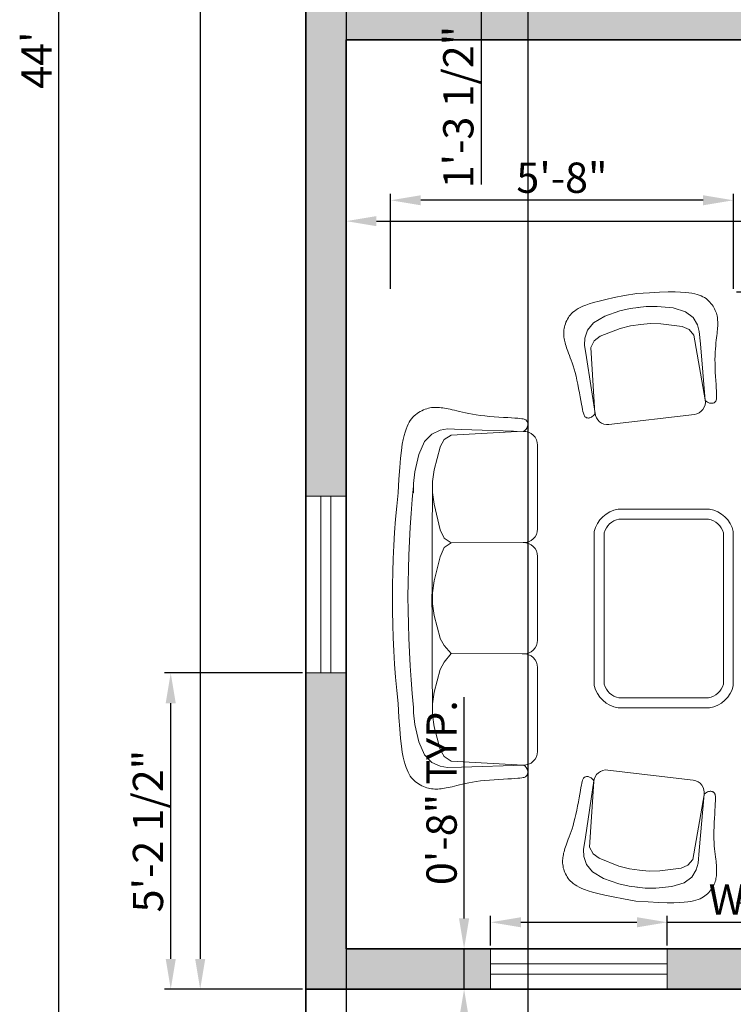
# Model space of a CAD drawing. Units: inches. Extents: x 2129 to 3258, y 1851 to 3021.
# Tile 2 of 10: x 2129 to 2271, y 1956 to 2151. Entities that reach past the tile are written whole.
import ezdxf

# ---------------------------------------------------------------- set-up
doc = ezdxf.new("R2010")
doc.units = ezdxf.units.IN
for name, color, linetype, lineweight in [('A-ANNO-DIMS', 2, 'Continuous', 18), ('A-FURN', 8, 'Continuous', 18), ('A-GLAZ', 4, 'Continuous', 18), ('A-WALL', 7, 'Continuous', 35)]:
    doc.layers.add(name, color=color, linetype=linetype, lineweight=lineweight)
doc.layers.add('A-WALL-PATT', color=32, linetype='Continuous', lineweight=13, true_color=0xcd6928)
doc.styles.get("Standard").update_dxf_attribs({"font": 'arial.ttf'})
doc.dimstyles.new('ISO-25', dxfattribs={"dimtxt": 6, "dimasz": 6, "dimexe": 1.25, "dimexo": 0.625, "dimtad": 1, "dimdec": 1, "dimlunit": 3, "dimtxsty": 'Standard', "dimcen": 2.5, "dimclrd": 5, "dimclre": 5, "dimadec": 0, "dimazin": 0, "dimtfac": 1, "dimtdec": 1, "dimtmove": 0, "dimatfit": 3, "dimfxl": 1, "dimarcsym": 0})

# ---------------------------------------------------------------- blocks, each defined once
blk = doc.blocks.new('sofa arrangement 10')
for p, q in [((-548, 1633.4), (-478.2, 1637.4)), ((651.3, 1633.4), (581.5, 1637.4)), ((-833.9, 1581.8), (-823.7, 1587.2)), ((-823.7, 1587.2), (-812.1, 1592.5)), ((-812.1, 1592.5), (-799.1, 1597.5)), ((-799.1, 1597.5), (-784.4, 1602.4)), ((-784.4, 1602.4), (-767.6, 1607.2)), ((-767.6, 1607.2), (-747.5, 1611.8)), ((-747.5, 1611.8), (-722.8, 1616.4)), ((-722.8, 1616.4), (-691.9, 1620.8)), ((-691.9, 1620.8), (-653.4, 1625.1)), ((-653.4, 1625.1), (-605.9, 1629.3)), ((-605.9, 1629.3), (-548, 1633.4)), ((709.2, 1629.3), (651.3, 1633.4)), ((756.7, 1625.1), (709.2, 1629.3)), ((795.2, 1620.8), (756.7, 1625.1)), ((826.1, 1616.4), (795.2, 1620.8)), ((850.9, 1611.8), (826.1, 1616.4)), ((870.9, 1607.2), (850.9, 1611.8)), ((887.7, 1602.4), (870.9, 1607.2)), ((902.4, 1597.5), (887.7, 1602.4)), ((915.5, 1592.5), (902.4, 1597.5)), ((927, 1587.2), (915.5, 1592.5)), ((937.2, 1581.8), (927, 1587.2)), ((-882.6, 1534.1), (-877.2, 1542)), ((-877.2, 1542), (-871.4, 1549.5)), ((-871.4, 1549.5), (-865.1, 1556.8)), ((-865.1, 1556.8), (-858.4, 1563.6)), ((-858.4, 1563.6), (-851.1, 1570)), ((-851.1, 1570), (-843, 1576)), ((-843, 1576), (-833.9, 1581.8)), ((-670.8, 1533.8), (-584, 1552.9)), ((-584, 1552.9), (-524.7, 1559.2)), ((-524.7, 1559.2), (-497.4, 1559.2)), ((628.1, 1559.2), (581.5, 1559.2)), ((607.1, 1559.2), (585.6, 1559.2)), ((687.3, 1552.9), (628.1, 1559.2)), ((774.1, 1533.8), (687.3, 1552.9)), ((946.3, 1576), (937.2, 1581.8)), ((954.4, 1570), (946.3, 1576)), ((961.8, 1563.6), (954.4, 1570)), ((968.5, 1556.8), (961.8, 1563.6)), ((974.8, 1549.5), (968.5, 1556.8)), ((980.6, 1542), (974.8, 1549.5)), ((985.9, 1534.1), (980.6, 1542)), ((-904.1, 1484.8), (-901.8, 1492.9)), ((-901.8, 1492.9), (-899, 1501.2)), ((-899, 1501.2), (-895.7, 1509.5)), ((-895.7, 1509.5), (-891.8, 1517.8)), ((-891.8, 1517.8), (-887.5, 1526)), ((-887.5, 1526), (-882.6, 1534.1)), ((-774.5, 1468.3), (-736.4, 1504.2)), ((-736.4, 1504.2), (-670.8, 1533.8)), ((839.7, 1504.2), (774.1, 1533.8)), ((877.8, 1468.3), (839.7, 1504.2)), ((990.8, 1526), (985.9, 1534.1)), ((995.2, 1517.8), (990.8, 1526)), ((999, 1509.5), (995.2, 1517.8)), ((1002.4, 1501.2), (999, 1509.5)), ((1005.2, 1492.9), (1002.4, 1501.2)), ((1007.4, 1484.8), (1005.2, 1492.9)), ((-908.3, 1445.1), (-908.2, 1453)), ((-908, 1437.2), (-908.3, 1445.1)), ((-908.2, 1453), (-907.8, 1460.9)), ((-907.5, 1429.1), (-908, 1437.2)), ((-907.8, 1460.9), (-907, 1468.8)), ((-907, 1468.8), (-905.8, 1476.8)), ((-905.8, 1476.8), (-904.1, 1484.8)), ((-793.5, 1426), (-774.5, 1468.3)), ((-594.6, 1455.6), (-708.9, 1426)), ((-535.3, 1464), (-594.6, 1455.6)), ((-478.2, 1464), (-535.3, 1464)), ((-421, 1455.6), (-480.3, 1464)), ((-480.3, 1464), (-478.2, 1464)), ((-306.7, 1426), (-421, 1455.6)), ((-149.4, 1426), (-35.1, 1455.6)), ((-35.1, 1455.6), (24.1, 1464)), ((24.1, 1464), (77.1, 1464)), ((77.1, 1464), (79.2, 1464)), ((79.2, 1464), (138.5, 1455.6)), ((138.5, 1455.6), (260.8, 1426)), ((896.9, 1426), (877.8, 1468.3)), ((1009.1, 1476.8), (1007.4, 1484.8)), ((1010.4, 1468.8), (1009.1, 1476.8)), ((1011.2, 1460.9), (1010.4, 1468.8)), ((1010.8, 1429.1), (1011.4, 1437.2)), ((1011.6, 1453), (1011.2, 1460.9)), ((1011.4, 1437.2), (1011.6, 1445.1)), ((1011.6, 1445.1), (1011.6, 1453)), ((-906.7, 1421), (-907.5, 1429.1)), ((-905.7, 1412.7), (-906.7, 1421)), ((-904.4, 1404.1), (-905.7, 1412.7)), ((-902.8, 1395.1), (-904.4, 1404.1)), ((-901, 1385.6), (-902.8, 1395.1)), ((-799.9, 1387.9), (-793.5, 1426)), ((-797.8, 1318.1), (-799.9, 1387.9)), ((-744.9, 1404.8), (-768.1, 1371)), ((-708.9, 1426), (-744.9, 1404.8)), ((-306.7, 1426), (-270.7, 1404.8)), ((-270.7, 1404.8), (-226.6, 1371)), ((-186.6, 1404.8), (-226.6, 1371)), ((-150.6, 1426), (-186.6, 1404.8)), ((260.8, 1426), (306.7, 1404.8)), ((813.4, 1426), (849.4, 1404.8)), ((849.4, 1404.8), (872.7, 1371)), ((849.4, 1404.8), (872.7, 1371)), ((903.2, 1387.9), (896.9, 1426)), ((901.1, 1318.1), (903.2, 1387.9)), ((1004.4, 1385.6), (1006.2, 1395.1)), ((1006.2, 1395.1), (1007.7, 1404.1)), ((1007.7, 1404.1), (1009, 1412.7)), ((1009, 1412.7), (1010, 1421)), ((1010, 1421), (1010.8, 1429.1)), ((-898.9, 1375.6), (-901, 1385.6)), ((-896.5, 1364.8), (-898.9, 1375.6)), ((-893.7, 1353.4), (-896.5, 1364.8)), ((-890.7, 1341), (-893.7, 1353.4)), ((-887.4, 1327.7), (-890.7, 1341)), ((-768.1, 1371), (-787.5, 1008.1)), ((-226.6, 1371), (-228.1, 1008.1)), ((-226.6, 1371), (-228.1, 1008.1)), ((872.7, 1371), (892.1, 1008.1)), ((990.7, 1327.7), (994, 1341)), ((994, 1341), (997.1, 1353.4)), ((997.1, 1353.4), (999.8, 1364.8)), ((999.8, 1364.8), (1002.2, 1375.6)), ((1002.2, 1375.6), (1004.4, 1385.6)), ((-883.9, 1313.4), (-887.4, 1327.7)), ((-880.4, 1297.9), (-883.9, 1313.4)), ((-876.9, 1281.2), (-880.4, 1297.9)), ((-787.6, 1004.4), (-797.8, 1318.1)), ((891, 1004.4), (901.1, 1318.1)), ((980.3, 1281.2), (983.7, 1297.9)), ((983.7, 1297.9), (987.3, 1313.4)), ((987.3, 1313.4), (990.7, 1327.7)), ((-873.6, 1263.2), (-876.9, 1281.2)), ((-870.4, 1243.8), (-873.6, 1263.2)), ((-867.6, 1222.9), (-870.4, 1243.8)), ((971, 1222.9), (973.8, 1243.8)), ((973.8, 1243.8), (976.9, 1263.2)), ((976.9, 1263.2), (980.3, 1281.2)), ((-865.2, 1200.6), (-867.6, 1222.9)), ((-863, 1177.2), (-865.2, 1200.6)), ((966.4, 1177.2), (968.5, 1200.6)), ((968.5, 1200.6), (971, 1222.9)), ((-861.2, 1153.4), (-863, 1177.2)), ((-859.7, 1129.8), (-861.2, 1153.4)), ((963, 1129.8), (964.6, 1153.4)), ((964.6, 1153.4), (966.4, 1177.2)), ((-858.3, 1107), (-859.7, 1129.8)), ((-857.1, 1085.6), (-858.3, 1107)), ((960.4, 1085.6), (961.7, 1107)), ((961.7, 1107), (963, 1129.8)), ((-856, 1066.1), (-857.1, 1085.6)), ((-854.9, 1049.1), (-856, 1066.1)), ((-853.9, 1035.2), (-854.9, 1049.1)), ((957.2, 1035.2), (958.3, 1049.1)), ((958.3, 1049.1), (959.3, 1066.1)), ((959.3, 1066.1), (960.4, 1085.6)), ((-852.8, 1024), (-853.9, 1035.2)), ((-851.7, 1015.2), (-852.8, 1024)), ((-850.5, 1008.5), (-851.7, 1015.2)), ((-849.3, 1003.4), (-850.5, 1008.5)), ((-848, 999.6), (-849.3, 1003.4)), ((-846.6, 996.8), (-848, 999.6)), ((-845, 994.5), (-846.6, 996.8)), ((-843.4, 992.5), (-845, 994.5)), ((-841.6, 990.7), (-843.4, 992.5)), ((-839.6, 989.1), (-841.6, 990.7)), ((-799.3, 993.5), (-804.6, 989.9)), ((-793.6, 998.3), (-799.3, 993.5)), ((-787.6, 1004.4), (-793.6, 998.3)), ((-786.9, 1011.2), (-787.4, 1011.2)), ((-787.4, 1010.4), (-786.9, 1011.2)), ((-229.1, 1010.4), (-228.7, 1011.2)), ((-228.7, 1011.2), (-229.1, 1011.2)), ((-228.7, 1011.2), (-228.2, 1011.2)), ((-228.2, 1010.4), (-228.7, 1011.2)), ((890.3, 1011.2), (890.7, 1011.2)), ((890.8, 1010.4), (890.3, 1011.2)), ((891, 1004.4), (897, 998.3)), ((897, 998.3), (902.6, 993.5)), ((902.6, 993.5), (907.9, 989.9)), ((942.9, 989.1), (944.9, 990.7)), ((944.9, 990.7), (946.7, 992.5)), ((946.7, 992.5), (948.4, 994.5)), ((948.4, 994.5), (949.9, 996.8)), ((949.9, 996.8), (951.3, 999.6)), ((951.3, 999.6), (952.6, 1003.4)), ((952.6, 1003.4), (953.9, 1008.5)), ((953.9, 1008.5), (955, 1015.2)), ((955, 1015.2), (956.1, 1024)), ((956.1, 1024), (957.2, 1035.2)), ((-837.4, 987.7), (-839.6, 989.1)), ((-834.9, 986.6), (-837.4, 987.7)), ((-832.2, 985.7), (-834.9, 986.6)), ((-829.3, 985), (-832.2, 985.7)), ((-826, 984.6), (-829.3, 985)), ((-822.4, 984.5), (-826, 984.6)), ((-818.4, 984.8), (-822.4, 984.5)), ((-814.2, 985.7), (-818.4, 984.8)), ((-809.6, 987.4), (-814.2, 985.7)), ((-804.6, 989.9), (-809.6, 987.4)), ((907.9, 989.9), (912.9, 987.4)), ((912.9, 987.4), (917.5, 985.7)), ((917.5, 985.7), (921.8, 984.8)), ((921.8, 984.8), (925.7, 984.5)), ((925.7, 984.5), (929.3, 984.6)), ((929.3, 984.6), (932.6, 985)), ((932.6, 985), (935.6, 985.7)), ((935.6, 985.7), (938.3, 986.6)), ((938.3, 986.6), (940.7, 987.7)), ((940.7, 987.7), (942.9, 989.1)), ((-718.5, 935.3), (-297.1, 935.3)), ((262.4, 935.3), (-159, 935.3)), ((-1335.3, 794.4), (-1343, 790.4)), ((-1327.5, 797.9), (-1335.3, 794.4)), ((-1319.6, 801), (-1327.5, 797.9)), ((-1311.7, 803.6), (-1319.6, 801)), ((-1303.8, 805.7), (-1311.7, 803.6)), ((-1296.1, 807.3), (-1303.8, 805.7)), ((-1288.5, 808.5), (-1296.1, 807.3)), ((-1281.1, 809.2), (-1288.5, 808.5)), ((-1273.7, 809.4), (-1281.1, 809.2)), ((-1266.5, 809.3), (-1273.7, 809.4)), ((-1259.4, 808.8), (-1266.5, 809.3)), ((-1252.2, 808), (-1259.4, 808.8)), ((-1245.1, 806.9), (-1252.2, 808)), ((-1237.9, 805.5), (-1245.1, 806.9)), ((-1230.6, 804), (-1237.9, 805.5)), ((-1223.2, 802.1), (-1230.6, 804)), ((-1215.6, 800.1), (-1223.2, 802.1)), ((-1207.6, 797.7), (-1215.6, 800.1)), ((-1199.3, 795), (-1207.6, 797.7)), ((-1190.4, 792), (-1199.3, 795)), ((1320.4, 792.1), (1328.3, 794.5)), ((1328.3, 794.5), (1336, 796.6)), ((1336, 796.6), (1343.4, 798.4)), ((1343.4, 798.4), (1350.6, 800)), ((1350.6, 800), (1357.8, 801.3)), ((1357.8, 801.3), (1365, 802.4)), ((1365, 802.4), (1372.1, 803.2)), ((1372.1, 803.2), (1379.3, 803.7)), ((1379.3, 803.7), (1386.5, 803.8)), ((1386.5, 803.8), (1393.8, 803.6)), ((1393.8, 803.6), (1401.3, 802.9)), ((1401.3, 802.9), (1408.8, 801.8)), ((1408.8, 801.8), (1416.6, 800.1)), ((1416.6, 800.1), (1424.5, 798)), ((1424.5, 798), (1432.4, 795.4)), ((1432.4, 795.4), (1440.3, 792.4)), ((-1389.6, 746.9), (-1395.6, 737.1)), ((-1383.6, 755.6), (-1389.6, 746.9)), ((-1377.4, 763.2), (-1383.6, 755.6)), ((-1371.1, 769.8), (-1377.4, 763.2)), ((-1364.5, 775.8), (-1371.1, 769.8)), ((-1357.6, 781.1), (-1364.5, 775.8)), ((-1350.5, 786), (-1357.6, 781.1)), ((-1343, 790.4), (-1350.5, 786)), ((-1181, 788.7), (-1190.4, 792)), ((-1171, 784.9), (-1181, 788.7)), ((-1160.1, 780.9), (-1171, 784.9)), ((-1148.5, 776.4), (-1160.1, 780.9)), ((-1135.9, 771.8), (-1148.5, 776.4)), ((-1122.4, 766.9), (-1135.9, 771.8)), ((-1107.7, 762), (-1122.4, 766.9)), ((-1091.8, 757), (-1107.7, 762)), ((-1074.6, 752.1), (-1091.8, 757)), ((-1056, 747.3), (-1074.6, 752.1)), ((-1036.1, 742.7), (-1056, 747.3)), ((1168.8, 741.7), (1187.4, 746.5)), ((1187.4, 746.5), (1204.5, 751.5)), ((1204.5, 751.5), (1220.4, 756.4)), ((1220.4, 756.4), (1235.1, 761.4)), ((1235.1, 761.4), (1248.7, 766.2)), ((1248.7, 766.2), (1261.3, 770.9)), ((1261.3, 770.9), (1272.9, 775.3)), ((1272.9, 775.3), (1283.7, 779.4)), ((1283.7, 779.4), (1293.8, 783.1)), ((1293.8, 783.1), (1303.2, 786.4)), ((1303.2, 786.4), (1312, 789.4)), ((1312, 789.4), (1320.4, 792.1)), ((1440.3, 792.4), (1448.1, 788.8)), ((1448.1, 788.8), (1455.8, 784.8)), ((1455.8, 784.8), (1463.2, 780.4)), ((1463.2, 780.4), (1470.4, 775.5)), ((1470.4, 775.5), (1477.3, 770.2)), ((1477.3, 770.2), (1483.8, 764.3)), ((1483.8, 764.3), (1490.2, 757.6)), ((1490.2, 757.6), (1496.3, 750)), ((1496.3, 750), (1502.4, 741.4)), ((-1413.7, 698.5), (-1420, 680.9)), ((-1407.6, 713.1), (-1413.7, 698.5)), ((-1401.6, 725.9), (-1407.6, 713.1)), ((-1395.6, 737.1), (-1401.6, 725.9)), ((-1247.3, 702.4), (-1287.6, 689.7)), ((-1212.3, 704), (-1247.3, 702.4)), ((-1149.5, 694.5), (-1212.3, 704)), ((-867.4, 651.5), (-1149.5, 694.5)), ((-1015.2, 738.3), (-1036.1, 742.7)), ((-994, 734.1), (-1015.2, 738.3)), ((-972.9, 730.1), (-994, 734.1)), ((-952.4, 726.4), (-972.9, 730.1)), ((-933.2, 723), (-952.4, 726.4)), ((-915.7, 719.9), (-933.2, 723)), ((-900.5, 717.1), (-915.7, 719.9)), ((-888.1, 714.6), (-900.5, 717.1)), ((-878.1, 712.5), (-888.1, 714.6)), ((-870.3, 710.5), (-878.1, 712.5)), ((-864.3, 708.7), (-870.3, 710.5)), ((-859.9, 707.1), (-864.3, 708.7)), ((-856.6, 705.5), (-859.9, 707.1)), ((-854.2, 703.9), (-856.6, 705.5)), ((-852.3, 702.3), (-854.2, 703.9)), ((-850.6, 700.6), (-852.3, 702.3)), ((-849.2, 698.7), (-850.6, 700.6)), ((-848, 696.8), (-849.2, 698.7)), ((-847, 694.6), (-848, 696.8)), ((-846.2, 692.3), (-847, 694.6)), ((962, 693.2), (963.4, 695)), ((963.4, 695), (965, 696.7)), ((965, 696.7), (966.9, 698.3)), ((966.9, 698.3), (969.3, 699.9)), ((969.3, 699.9), (972.6, 701.5)), ((972.6, 701.5), (977.1, 703.2)), ((977.1, 703.2), (983, 704.9)), ((983, 704.9), (990.8, 706.9)), ((990.8, 706.9), (1000.8, 709.1)), ((1000.8, 709.1), (1013.3, 711.5)), ((1013.3, 711.5), (1028.5, 714.3)), ((1028.5, 714.3), (1045.9, 717.4)), ((1045.9, 717.4), (1065.2, 720.8)), ((1065.2, 720.8), (1085.6, 724.5)), ((1085.6, 724.5), (1106.7, 728.5)), ((1106.7, 728.5), (1128, 732.7)), ((1128, 732.7), (1148.9, 737.1)), ((1148.9, 737.1), (1168.8, 741.7)), ((1262.2, 689), (1325, 698.4)), ((1325, 698.4), (1360.1, 696.8)), ((1360.1, 696.8), (1400.3, 684.2)), ((1502.4, 741.4), (1508.4, 731.5)), ((1508.4, 731.5), (1514.3, 720.3)), ((1514.3, 720.3), (1520.3, 707.5)), ((1520.3, 707.5), (1526.4, 692.9)), ((-1426.8, 659), (-1434.1, 631.6)), ((-1420, 680.9), (-1426.8, 659)), ((-1324.1, 659.2), (-1357.9, 603.2)), ((-1287.6, 689.7), (-1324.1, 659.2)), ((-1256.4, 625.9), (-1233.5, 656.1)), ((-1233.5, 656.1), (-1200.4, 673.5)), ((-1200.4, 673.5), (-870.8, 651.8)), ((-873.7, 651.6), (-873.6, 652)), ((-872.9, 652), (-873.7, 651.6)), ((-867.4, 651.5), (-861.2, 656.3)), ((-861.2, 656.3), (-856.3, 660.9)), ((-856.3, 660.9), (-852.5, 665.3)), ((-852.5, 665.3), (-849.7, 669.5)), ((-849.7, 669.5), (-847.7, 673.5)), ((-847.7, 673.5), (-846.4, 677.2)), ((-846.4, 677.2), (-845.7, 680.8)), ((-845.7, 689.8), (-846.2, 692.3)), ((-845.4, 687), (-845.7, 689.8)), ((-845.7, 680.8), (-845.4, 684)), ((-845.4, 684), (-845.4, 687)), ((958.2, 681.5), (958.5, 684.2)), ((958.2, 678.5), (958.2, 681.5)), ((958.5, 675.2), (958.2, 678.5)), ((958.5, 684.2), (959, 686.7)), ((959.2, 671.7), (958.5, 675.2)), ((959, 686.7), (959.7, 689.1)), ((960.5, 667.9), (959.2, 671.7)), ((959.7, 689.1), (960.7, 691.2)), ((962.4, 663.9), (960.5, 667.9)), ((960.7, 691.2), (962, 693.2)), ((965.2, 659.7), (962.4, 663.9)), ((969, 655.3), (965.2, 659.7)), ((974, 650.7), (969, 655.3)), ((980.2, 646), (974, 650.7)), ((980.2, 646), (1262.2, 689)), ((1313.2, 667.9), (983.5, 646.3)), ((985.6, 646.4), (986.4, 646.1)), ((986.4, 646.1), (986.4, 646.5)), ((1346.2, 650.6), (1313.2, 667.9)), ((1369.2, 620.4), (1346.2, 650.6)), ((1400.3, 684.2), (1436.9, 653.6)), ((1436.9, 653.6), (1470.7, 597.6)), ((1526.4, 692.9), (1532.8, 675.3)), ((1532.8, 675.3), (1539.6, 653.4)), ((1539.6, 653.4), (1546.9, 626)), ((-1442.2, 597.3), (-1451.1, 554.9)), ((-1434.1, 631.6), (-1442.2, 597.3)), ((-1357.9, 603.2), (-1384.5, 526.9)), ((-1295.5, 526), (-1256.4, 625.9)), ((1408.3, 520.4), (1369.2, 620.4)), ((1470.7, 597.6), (1497.2, 521.3)), ((1546.9, 626), (1554.9, 591.7)), ((-1451.1, 554.9), (-1461.1, 503.1)), ((-812.5, 581.7), (-863.9, 151.6)), ((925.2, 576.1), (976.6, 146.1)), ((1554.9, 591.7), (1563.9, 549.3)), ((1563.9, 549.3), (1573.8, 497.5)), ((-1461.1, 503.1), (-1472.2, 440.5)), ((-1384.5, 526.9), (-1396.6, 474.1)), ((-1309.5, 473.4), (-1295.5, 526)), ((1422.3, 467.8), (1408.3, 520.4)), ((1497.2, 521.3), (1509.4, 468.5)), ((1573.8, 497.5), (1584.9, 434.9)), ((-1396.6, 474.1), (-1401.6, 432.1)), ((-1315.7, 421.8), (-1309.5, 473.4)), ((1428.5, 416.2), (1422.3, 467.8)), ((1509.4, 468.5), (1514.4, 426.5)), ((-1476, 378.3), (-1472.2, 440.5)), ((-1406.2, 393.7), (-1401.2, 435.7)), ((-1321.4, 374), (-1315.7, 421.8)), ((1434.2, 368.5), (1428.5, 416.2)), ((1519, 388.1), (1513.9, 430.2)), ((1588.7, 372.7), (1584.9, 434.9)), ((-1478.4, 326.5), (-1476, 378.3)), ((-1406.9, 339.5), (-1406.2, 393.7)), ((-1320.2, 319.6), (-1321.4, 374)), ((1432.9, 314.1), (1434.2, 368.5)), ((1519.6, 334), (1519, 388.1)), ((1591.2, 320.9), (1588.7, 372.7)), ((-1479.7, 283.8), (-1478.4, 326.5)), ((-1399.1, 259.2), (-1406.9, 339.5)), ((-1305.8, 213.3), (-1320.2, 319.6)), ((1418.5, 207.7), (1432.9, 314.1)), ((1511.8, 253.6), (1519.6, 334)), ((1592.4, 278.2), (1591.2, 320.9)), ((-1479.9, 249.1), (-1479.7, 283.8)), ((-1479.2, 220.9), (-1479.9, 249.1)), ((-1379.4, 196.7), (-1399.1, 259.2)), ((1492.2, 191.2), (1511.8, 253.6)), ((1592.6, 243.5), (1592.4, 278.2)), ((-1477.7, 198.2), (-1479.2, 220.9)), ((-1475.7, 179.7), (-1477.7, 198.2)), ((-1290.6, 178.5), (-1305.8, 213.3)), ((1403.3, 172.9), (1418.5, 207.7)), ((1590.5, 192.7), (1591.9, 215.4)), ((1591.9, 215.4), (1592.6, 243.5)), ((-1473.2, 164), (-1475.7, 179.7)), ((-1470.4, 150.2), (-1473.2, 164)), ((-1467.2, 137.9), (-1470.4, 150.2)), ((-1351.1, 158.5), (-1379.4, 196.7)), ((-1314.9, 136.7), (-1351.1, 158.5)), ((-1262.5, 153.8), (-1290.6, 178.5)), ((-937.1, 97.2), (-1262.5, 153.8)), ((1375.3, 148.3), (1403.3, 172.9)), ((1427.7, 131.1), (1463.8, 152.9)), ((1463.8, 152.9), (1492.2, 191.2)), ((1583.1, 144.6), (1586, 158.4)), ((1586, 158.4), (1588.4, 174.1)), ((1588.4, 174.1), (1590.5, 192.7)), ((-1463.7, 126.9), (-1467.2, 137.9)), ((-1459.9, 117.1), (-1463.7, 126.9)), ((-1455.7, 108.3), (-1459.9, 117.1)), ((-1451.1, 100.3), (-1455.7, 108.3)), ((-1446.1, 93), (-1451.1, 100.3)), ((-1281.3, 126.9), (-1314.9, 136.7)), ((-1218, 121.2), (-1281.3, 126.9)), ((-933.8, 96.5), (-1218, 121.2)), ((1046.5, 91), (1330.8, 115.7)), ((1049.8, 91.6), (1375.3, 148.3)), ((1330.8, 115.7), (1394, 121.3)), ((1394, 121.3), (1427.7, 131.1)), ((1563.9, 94.7), (1568.5, 102.7)), ((1568.5, 102.7), (1572.7, 111.5)), ((1572.7, 111.5), (1576.5, 121.3)), ((1576.5, 121.3), (1580, 132.3)), ((1580, 132.3), (1583.1, 144.6)), ((-1440.7, 86.2), (-1446.1, 93)), ((-1434.9, 79.7), (-1440.7, 86.2)), ((-1428.7, 73.7), (-1434.9, 79.7)), ((-1422.2, 68), (-1428.7, 73.7)), ((-1415.4, 62.7), (-1422.2, 68)), ((-1408.4, 57.9), (-1415.4, 62.7)), ((-1401.4, 53.5), (-1408.4, 57.9)), ((-1394.2, 49.6), (-1401.4, 53.5)), ((-1387.1, 46.2), (-1394.2, 49.6)), ((-933.8, 96.5), (-928.9, 90.5)), ((-928.9, 90.5), (-925.1, 84.8)), ((-924.1, 49.9), (-925.5, 48)), ((-925.1, 84.8), (-922.5, 79.7)), ((-922.8, 51.9), (-924.1, 49.9)), ((-921.7, 54.3), (-922.8, 51.9)), ((-922.5, 79.7), (-920.7, 74.9)), ((-920.8, 56.9), (-921.7, 54.3)), ((-920.1, 59.8), (-920.8, 56.9)), ((-920.7, 74.9), (-919.8, 70.6)), ((-919.6, 63), (-920.1, 59.8)), ((-919.8, 70.6), (-919.4, 66.6)), ((-919.4, 66.6), (-919.6, 63)), ((1032.5, 65), (1032.2, 61)), ((1032.2, 61), (1032.3, 57.5)), ((1032.3, 57.5), (1032.8, 54.2)), ((1033.5, 69.3), (1032.5, 65)), ((1032.8, 54.2), (1033.5, 51.3)), ((1035.2, 74.1), (1033.5, 69.3)), ((1033.5, 51.3), (1034.4, 48.7)), ((1037.9, 79.3), (1035.2, 74.1)), ((1041.6, 84.9), (1037.9, 79.3)), ((1046.5, 91), (1041.6, 84.9)), ((1514.1, 47.9), (1521.2, 52.3)), ((1521.2, 52.3), (1528.2, 57.2)), ((1528.2, 57.2), (1534.9, 62.4)), ((1534.9, 62.4), (1541.4, 68.1)), ((1541.4, 68.1), (1547.6, 74.2)), ((1547.6, 74.2), (1553.5, 80.6)), ((1553.5, 80.6), (1558.9, 87.4)), ((1558.9, 87.4), (1563.9, 94.7)), ((-1380, 43.3), (-1387.1, 46.2)), ((-1372.9, 40.9), (-1380, 43.3)), ((-1365.9, 38.9), (-1372.9, 40.9)), ((-1358.8, 37.3), (-1365.9, 38.9)), ((-1351.7, 36.1), (-1358.8, 37.3)), ((-1344.6, 35.2), (-1351.7, 36.1)), ((-1337.4, 34.6), (-1344.6, 35.2)), ((-1330.1, 34.2), (-1337.4, 34.6)), ((-1322.7, 34), (-1330.1, 34.2)), ((-1315, 34.1), (-1322.7, 34)), ((-1307.1, 34.3), (-1315, 34.1)), ((-1298.8, 34.7), (-1307.1, 34.3)), ((-1290.1, 35.3), (-1298.8, 34.7)), ((-1280.8, 36.2), (-1290.1, 35.3)), ((-1270.9, 37.2), (-1280.8, 36.2)), ((-1260.2, 38.4), (-1270.9, 37.2)), ((-1248.7, 39.9), (-1260.2, 38.4)), ((-1236.4, 41.4), (-1248.7, 39.9)), ((-1223.1, 43), (-1236.4, 41.4)), ((-1208.7, 44.5), (-1223.1, 43)), ((-1193.3, 45.8), (-1208.7, 44.5)), ((-1176.7, 46.9), (-1193.3, 45.8)), ((-1158.8, 47.6), (-1176.7, 46.9)), ((-1139.6, 47.9), (-1158.8, 47.6)), ((-1119.2, 47.7), (-1139.6, 47.9)), ((-1097.9, 47.1), (-1119.2, 47.7)), ((-1076.2, 46.2), (-1097.9, 47.1)), ((-1054.7, 45), (-1076.2, 46.2)), ((-1034, 43.8), (-1054.7, 45)), ((-1014.5, 42.6), (-1034, 43.8)), ((-996.8, 41.5), (-1014.5, 42.6)), ((-981.4, 40.6), (-996.8, 41.5)), ((-968.7, 40.1), (-981.4, 40.6)), ((-958.5, 39.9), (-968.7, 40.1)), ((-950.4, 39.9), (-958.5, 39.9)), ((-944.2, 40.2), (-950.4, 39.9)), ((-939.5, 40.8), (-944.2, 40.2)), ((-936, 41.6), (-939.5, 40.8)), ((-933.2, 42.5), (-936, 41.6)), ((-931, 43.7), (-933.2, 42.5)), ((-929, 44.9), (-931, 43.7)), ((-927.2, 46.4), (-929, 44.9)), ((-925.5, 48), (-927.2, 46.4)), ((1034.4, 48.7), (1035.5, 46.4)), ((1035.5, 46.4), (1036.8, 44.3)), ((1036.8, 44.3), (1038.3, 42.4)), ((1038.3, 42.4), (1039.9, 40.8)), ((1039.9, 40.8), (1041.8, 39.4)), ((1041.8, 39.4), (1043.8, 38.1)), ((1043.8, 38.1), (1046, 37)), ((1046, 37), (1048.7, 36)), ((1048.7, 36), (1052.3, 35.2)), ((1052.3, 35.2), (1057, 34.7)), ((1057, 34.7), (1063.2, 34.3)), ((1063.2, 34.3), (1071.2, 34.3)), ((1071.2, 34.3), (1081.4, 34.5)), ((1081.4, 34.5), (1094.2, 35.1)), ((1094.2, 35.1), (1109.6, 35.9)), ((1109.6, 35.9), (1127.3, 37)), ((1127.3, 37), (1146.8, 38.2)), ((1146.8, 38.2), (1167.5, 39.5)), ((1167.5, 39.5), (1189, 40.6)), ((1189, 40.6), (1210.6, 41.5)), ((1210.6, 41.5), (1231.9, 42.2)), ((1231.9, 42.2), (1252.4, 42.4)), ((1252.4, 42.4), (1271.6, 42.1)), ((1271.6, 42.1), (1289.4, 41.3)), ((1289.4, 41.3), (1306, 40.2)), ((1306, 40.2), (1321.5, 38.9)), ((1321.5, 38.9), (1335.8, 37.4)), ((1335.8, 37.4), (1349.1, 35.8)), ((1349.1, 35.8), (1361.5, 34.3)), ((1361.5, 34.3), (1372.9, 32.9)), ((1372.9, 32.9), (1383.6, 31.6)), ((1383.6, 31.6), (1393.5, 30.6)), ((1393.5, 30.6), (1402.8, 29.8)), ((1402.8, 29.8), (1411.6, 29.1)), ((1411.6, 29.1), (1419.9, 28.7)), ((1419.9, 28.7), (1427.8, 28.5)), ((1427.8, 28.5), (1435.4, 28.5)), ((1435.4, 28.5), (1442.8, 28.6)), ((1442.8, 28.6), (1450.1, 29)), ((1450.1, 29), (1457.3, 29.6)), ((1457.3, 29.6), (1464.5, 30.5)), ((1464.5, 30.5), (1471.6, 31.7)), ((1471.6, 31.7), (1478.6, 33.3)), ((1478.6, 33.3), (1485.7, 35.3)), ((1485.7, 35.3), (1492.7, 37.7)), ((1492.7, 37.7), (1499.8, 40.6)), ((1499.8, 40.6), (1507, 44)), ((1507, 44), (1514.1, 47.9))]:
    blk.add_line(p, q)
for points in [[(-478.2, 1637.4, -0.05358), (581.5, 1637.4, 12.163767)], [(-497.4, 1559.2, -0.050936), (617.3, 1559.2, 12.167348)], [(585.8, 1464, 0.004989), (-506.8, 1464, 0.847003)], [(331.4, 1008.1), (330, 1371), (331.4, 1008.1, 0.429937), (400.4, 935.3), (821.9, 935.3, 0.429937), (890.9, 1008.1)]]:
    blk.add_lwpolyline(points, format="xyb")
blk.add_lwpolyline([(812.2, 1426), (697.9, 1455.6), (638.7, 1464), (585.8, 1464), (583.6, 1464), (524.4, 1455.6), (396, 1426), (353.2, 1404.8), (330, 1371), (306.7, 1404.8)])
for points in [[(387.1, -50), (-387.1, -50, -0.304542), (-500, 69.8), (-500, 530.2, -0.304542), (-387.1, 650), (387.1, 650, -0.304542), (500, 530.2), (500, 69.8, -0.304542)], [(380.9, 0), (-380.9, 0, -0.280233), (-450, 74.4), (-450, 525.6, -0.280233), (-380.9, 600), (380.9, 600, -0.280233), (450, 525.6), (450, 74.4, -0.280233)]]:
    blk.add_lwpolyline(points, format="xyb", close=True)
for centre, radius, start, end in [((-718.5, 1004.4), 69.1, 176.9413, 270), ((-297.1, 1004.4), 69.1, 270, 3.0587), ((-297.1, 1004.4), 69.1, 270, 3.0587), ((-297.1, 1004.4), 69.1, 270, 3.0587), ((-159, 1004.4), 69.1, 176.9413, 270), ((-159, 1004.4), 69.1, 176.9413, 270), ((262.4, 1004.4), 69.1, 270, 3.0587), ((-874.9, 589.1), 62.8, 353.1831, 86.2418), ((987.6, 583.6), 62.8, 93.7582, 186.8169), ((-926.3, 159.1), 62.8, 260.1245, 353.1831), ((1039, 153.5), 62.8, 186.8169, 279.8755)]:
    blk.add_arc(centre, radius, start, end)
blk = doc.blocks.new('*D5')
at = {"layer": 'A-ANNO-DIMS', "color": 0, "lineweight": -2, "transparency": 16777216}
for p, q in [((2185.3, 2407.23), (2163.77, 2407.23)), ((2165.02, 2401.23), (2165.02, 1965.23)), ((2185.3, 1959.23), (2163.77, 1959.23))]:
    blk.add_line(p, q, dxfattribs=at)
at = {"layer": 'A-ANNO-DIMS', "color": 0, "transparency": 16777216}
for points in [[(2164.02, 2401.23), (2166.02, 2401.23), (2165.02, 2407.23)], [(2164.02, 1965.23), (2166.02, 1965.23), (2165.02, 1959.23)]]:
    blk.add_solid(points, dxfattribs=at)
at = {"layer": 'Defpoints', "color": 0, "transparency": 16777216}
for p in [(2185.93, 2407.23), (2165.02, 1959.23), (2185.93, 1959.23)]:
    blk.add_point(p, dxfattribs=at)
at = {"layer": 'A-ANNO-DIMS', "color": 0, "transparency": 16777216, "insert": (2161.33, 2183.23), "char_height": 6, "attachment_point": 5, "rotation": 90}
blk.add_mtext('37\'-4"', dxfattribs=at)
blk = doc.blocks.new('*D6')
at = {"layer": 'A-ANNO-DIMS', "color": 0, "lineweight": -2, "transparency": 16777216}
for p, q in [((2185.3, 2407.23), (2135.71, 2407.23)), ((2136.96, 2401.23), (2136.96, 1885.23)), ((2185.3, 1879.23), (2135.71, 1879.23))]:
    blk.add_line(p, q, dxfattribs=at)
at = {"layer": 'A-ANNO-DIMS', "color": 0, "transparency": 16777216}
for points in [[(2135.96, 2401.23), (2137.96, 2401.23), (2136.96, 2407.23)], [(2135.96, 1885.23), (2137.96, 1885.23), (2136.96, 1879.23)]]:
    blk.add_solid(points, dxfattribs=at)
at = {"layer": 'Defpoints', "color": 0, "transparency": 16777216}
for p in [(2185.93, 2407.23), (2136.96, 1879.23), (2185.93, 1879.23)]:
    blk.add_point(p, dxfattribs=at)
at = {"layer": 'A-ANNO-DIMS', "color": 0, "transparency": 16777216, "insert": (2133.34, 2143.23), "char_height": 6, "attachment_point": 5, "rotation": 90}
blk.add_mtext("44'", dxfattribs=at)
blk = doc.blocks.new('*D9')
at = {"layer": 'A-ANNO-DIMS', "color": 0, "lineweight": -2, "transparency": 16777216}
for p, q in [((2193.93, 2115.34), (2193.93, 2110.09)), ((2385.93, 2113.61), (2385.93, 2110.09)), ((2199.93, 2111.34), (2379.93, 2111.34))]:
    blk.add_line(p, q, dxfattribs=at)
at = {"layer": 'A-ANNO-DIMS', "color": 0, "transparency": 16777216}
for points in [[(2199.93, 2112.34), (2199.93, 2110.34), (2193.93, 2111.34)], [(2379.93, 2112.34), (2379.93, 2110.34), (2385.93, 2111.34)]]:
    blk.add_solid(points, dxfattribs=at)
at = {"layer": 'Defpoints', "color": 0, "transparency": 16777216}
for p in [(2193.93, 2115.96), (2385.93, 2114.23), (2385.93, 2111.34)]:
    blk.add_point(p, dxfattribs=at)
at = {"layer": 'A-ANNO-DIMS', "color": 0, "transparency": 16777216, "insert": (2289.93, 2115.03), "char_height": 6, "attachment_point": 5}
blk.add_mtext("16'", dxfattribs=at)
blk = doc.blocks.new('WIN-PLAN-35')
for p, q in [((0, 5), (35, 5)), ((0, 3), (35, 3))]:
    blk.add_line(p, q)
blk.add_lwpolyline([(0, 8), (35, 8), (35, 0), (0, 0)], close=True)
blk = doc.blocks.new('*D62')
at = {"layer": 'A-ANNO-DIMS', "color": 5, "lineweight": -2, "transparency": 16777216}
for p, q in [((2222.56, 1967.86), (2222.56, 1973.73)), ((2257.56, 1967.86), (2257.56, 1973.73)), ((2228.56, 1972.48), (2251.56, 1972.48)), ((2257.56, 1972.48), (2345.4, 1972.48))]:
    blk.add_line(p, q, dxfattribs=at)
at = {"layer": 'A-ANNO-DIMS', "color": 5, "transparency": 16777216}
for points in [[(2228.56, 1973.48), (2228.56, 1971.48), (2222.56, 1972.48)], [(2251.56, 1973.48), (2251.56, 1971.48), (2257.56, 1972.48)]]:
    blk.add_solid(points, dxfattribs=at)
at = {"layer": 'Defpoints', "color": 0, "transparency": 16777216}
for p in [(2257.56, 1972.48), (2222.56, 1967.23), (2257.56, 1967.23)]:
    blk.add_point(p, dxfattribs=at)
at = {"layer": 'A-ANNO-DIMS', "color": 0, "transparency": 16777216, "insert": (2304.48, 1976.21), "char_height": 6, "attachment_point": 5}
blk.add_mtext('WINDOW 2\'-11" TYP.', dxfattribs=at)
blk = doc.blocks.new('*D63')
at = {"layer": 'A-ANNO-DIMS', "color": 5, "lineweight": -2, "transparency": 16777216}
for p, q in [((2217.31, 1973.23), (2217.31, 2017.06)), ((2221.94, 1967.23), (2216.06, 1967.23)), ((2217.31, 1959.23), (2217.31, 1967.23)), ((2221.94, 1959.23), (2216.06, 1959.23)), ((2217.31, 1953.23), (2217.31, 1947.23))]:
    blk.add_line(p, q, dxfattribs=at)
at = {"layer": 'A-ANNO-DIMS', "color": 5, "transparency": 16777216}
for points in [[(2216.31, 1973.23), (2218.31, 1973.23), (2217.31, 1967.23)], [(2216.31, 1953.23), (2218.31, 1953.23), (2217.31, 1959.23)]]:
    blk.add_solid(points, dxfattribs=at)
at = {"layer": 'Defpoints', "color": 0, "transparency": 16777216}
for p in [(2217.31, 1967.23), (2222.56, 1967.23), (2222.56, 1959.23)]:
    blk.add_point(p, dxfattribs=at)
at = {"layer": 'A-ANNO-DIMS', "color": 0, "transparency": 16777216, "insert": (2213.63, 1998.15), "char_height": 6, "attachment_point": 5, "rotation": 90}
blk.add_mtext('0\'-8" TYP.', dxfattribs=at)
blk = doc.blocks.new('*D76')
at = {"layer": 'A-ANNO-DIMS', "color": 5, "lineweight": -2, "transparency": 16777216}
for p, q in [((2271.29, 2097.32), (2290.06, 2097.32)), ((2288.81, 1982.36), (2288.81, 2091.32)), ((2271.29, 1976.36), (2290.06, 1976.36))]:
    blk.add_line(p, q, dxfattribs=at)
at = {"layer": 'A-ANNO-DIMS', "color": 5, "transparency": 16777216}
for points in [[(2287.81, 2091.32), (2289.81, 2091.32), (2288.81, 2097.32)], [(2287.81, 1982.36), (2289.81, 1982.36), (2288.81, 1976.36)]]:
    blk.add_solid(points, dxfattribs=at)
at = {"layer": 'Defpoints', "color": 0, "transparency": 16777216}
for p in [(2270.67, 2097.32), (2288.81, 2097.32), (2270.67, 1976.36)]:
    blk.add_point(p, dxfattribs=at)
at = {"layer": 'A-ANNO-DIMS', "color": 0, "transparency": 16777216, "insert": (2285.08, 2036.84), "char_height": 6, "attachment_point": 5, "rotation": 90}
blk.add_mtext('SOFA GROUP 10\'-1"', dxfattribs=at)
blk = doc.blocks.new('*D77')
at = {"layer": 'A-ANNO-DIMS', "color": 5, "lineweight": -2, "transparency": 16777216}
for p, q in [((2202.74, 2097.95), (2202.74, 2116.72)), ((2270.67, 2097.95), (2270.67, 2116.72)), ((2264.67, 2115.47), (2208.74, 2115.47))]:
    blk.add_line(p, q, dxfattribs=at)
at = {"layer": 'A-ANNO-DIMS', "color": 5, "transparency": 16777216}
for points in [[(2208.74, 2116.47), (2208.74, 2114.47), (2202.74, 2115.47)], [(2264.67, 2116.47), (2264.67, 2114.47), (2270.67, 2115.47)]]:
    blk.add_solid(points, dxfattribs=at)
at = {"layer": 'Defpoints', "color": 0, "transparency": 16777216}
for p in [(2202.74, 2115.47), (2202.74, 2097.32), (2270.67, 2097.32)]:
    blk.add_point(p, dxfattribs=at)
at = {"layer": 'A-ANNO-DIMS', "color": 0, "transparency": 16777216, "insert": (2236.71, 2119.16), "char_height": 6, "attachment_point": 5}
blk.add_mtext('5\'-8"', dxfattribs=at)
blk = doc.blocks.new('*D97')
at = {"layer": 'A-ANNO-DIMS', "color": 5, "lineweight": -2, "transparency": 16777216}
for p, q in [((2193.93, 2272.48), (2193.93, 1851.23)), ((2229.93, 2272.48), (2229.93, 1851.23)), ((2199.93, 1852.48), (2223.93, 1852.48))]:
    blk.add_line(p, q, dxfattribs=at)
at = {"layer": 'A-ANNO-DIMS', "color": 5, "transparency": 16777216}
for points in [[(2199.93, 1853.48), (2199.93, 1851.48), (2193.93, 1852.48)], [(2223.93, 1853.48), (2223.93, 1851.48), (2229.93, 1852.48)]]:
    blk.add_solid(points, dxfattribs=at)
at = {"layer": 'Defpoints', "color": 0, "transparency": 16777216}
for p in [(2193.93, 2273.1), (2229.93, 2273.1), (2229.93, 1852.48)]:
    blk.add_point(p, dxfattribs=at)
at = {"layer": 'A-ANNO-DIMS', "color": 0, "transparency": 16777216, "insert": (2211.93, 1856.18), "char_height": 6, "attachment_point": 5}
blk.add_mtext('3\'-0"', dxfattribs=at)
blk = doc.blocks.new('*D110')
at = {"layer": 'A-ANNO-DIMS', "color": 5, "lineweight": -2, "transparency": 16777216}
for p, q in [((2194.55, 2170.77), (2221.93, 2170.77)), ((2220.68, 2164.77), (2220.68, 2161.23)), ((2194.55, 2155.23), (2221.93, 2155.23)), ((2220.68, 2155.23), (2220.68, 2118.62))]:
    blk.add_line(p, q, dxfattribs=at)
at = {"layer": 'A-ANNO-DIMS', "color": 5, "transparency": 16777216}
for points in [[(2219.68, 2164.77), (2221.68, 2164.77), (2220.68, 2170.77)], [(2219.68, 2161.23), (2221.68, 2161.23), (2220.68, 2155.23)]]:
    blk.add_solid(points, dxfattribs=at)
at = {"layer": 'Defpoints', "color": 0, "transparency": 16777216}
for p in [(2193.93, 2170.77), (2193.93, 2155.23), (2220.68, 2155.23)]:
    blk.add_point(p, dxfattribs=at)
at = {"layer": 'A-ANNO-DIMS', "color": 0, "transparency": 16777216, "insert": (2216.95, 2133.93), "char_height": 6, "attachment_point": 5, "rotation": 90}
blk.add_mtext('1\'-3 1/2"', dxfattribs=at)
blk = doc.blocks.new('*D111')
at = {"layer": 'A-ANNO-DIMS', "color": 5, "lineweight": -2, "transparency": 16777216}
for p, q in [((2185.3, 2021.85), (2157.93, 2021.85)), ((2159.18, 1965.23), (2159.18, 2015.85)), ((2185.3, 1959.23), (2157.93, 1959.23))]:
    blk.add_line(p, q, dxfattribs=at)
at = {"layer": 'A-ANNO-DIMS', "color": 5, "transparency": 16777216}
for points in [[(2158.18, 2015.85), (2160.18, 2015.85), (2159.18, 2021.85)], [(2158.18, 1965.23), (2160.18, 1965.23), (2159.18, 1959.23)]]:
    blk.add_solid(points, dxfattribs=at)
at = {"layer": 'Defpoints', "color": 0, "transparency": 16777216}
for p in [(2159.18, 2021.85), (2185.93, 2021.85), (2185.93, 1959.23)]:
    blk.add_point(p, dxfattribs=at)
at = {"layer": 'A-ANNO-DIMS', "color": 0, "transparency": 16777216, "insert": (2155.45, 1990.54), "char_height": 6, "attachment_point": 5, "rotation": 90}
blk.add_mtext('5\'-2 1/2"', dxfattribs=at)

msp = doc.modelspace()

# ---------------------------------------------------------------- hatches: boundary and pattern name
at = {"layer": 'A-WALL-PATT'}
h = msp.add_hatch(color=256, dxfattribs=at)
h.dxf.hatch_style = 1
h.paths.add_polyline_path([(2393.39, 2407.23), (2185.93, 2407.23), (2185.93, 2394.06), (2193.93, 2394.06), (2193.93, 2399.23), (2361.93, 2399.23), (2361.93, 2355.23), (2361.93, 2347.23), (2361.93, 2258.25), (2369.93, 2258.25), (2369.93, 2307.23), (2429.93, 2307.23), (2429.93, 2303.23), (2437.93, 2303.23), (2437.93, 2327.23), (2429.93, 2327.23), (2429.93, 2315.23), (2369.93, 2315.23), (2369.93, 2399.23), (2393.39, 2399.23)])
h.paths.add_polyline_path([(2569.93, 2407.23), (2410.42, 2407.23), (2410.42, 2399.23), (2429.93, 2399.23), (2429.93, 2351.23), (2437.93, 2351.23), (2437.93, 2399.23), (2561.93, 2399.23), (2561.93, 2317.22), (2569.93, 2317.22)])
h.paths.add_polyline_path([(2569.93, 2282.22), (2561.93, 2282.22), (2561.93, 2243.23), (2437.93, 2243.23), (2437.93, 2249.23), (2429.93, 2249.23), (2429.93, 2235.23), (2561.93, 2235.23), (2561.93, 2155.23), (2379.93, 2155.23), (2379.93, 2147.23), (2385.93, 2147.23), (2385.93, 2141.23), (2393.93, 2141.23), (2393.93, 2147.23), (2469.93, 2147.23), (2469.93, 2111.23), (2477.93, 2111.23), (2477.93, 2147.23), (2561.93, 2147.23), (2561.93, 2129.53), (2569.93, 2129.53)])
h.paths.add_polyline_path([(2569.93, 2112.5), (2561.93, 2112.5), (2561.93, 2063.23), (2477.93, 2063.23), (2477.93, 2069.23), (2469.93, 2069.23), (2469.93, 2063.23), (2445.93, 2063.23), (2445.93, 2055.23), (2561.93, 2055.23), (2561.93, 1951.04), (2569.93, 1951.04)])
h.paths.add_polyline_path([(2569.93, 1916.04), (2561.93, 1916.04), (2561.93, 1887.23), (2393.93, 1887.23), (2393.93, 2055.23), (2399.93, 2055.23), (2399.93, 2063.23), (2393.93, 2063.23), (2393.93, 2087.23), (2385.93, 2087.23), (2385.93, 1887.23), (2385.93, 1879.23), (2569.93, 1879.23)])
h.paths.add_polyline_path([(2193.93, 2147.23), (2289.93, 2147.23), (2289.93, 2155.23), (2193.93, 2155.23), (2193.93, 2170.77), (2185.93, 2170.77), (2185.93, 2056.85), (2193.93, 2056.85)])
h.paths.add_polyline_path([(2193.93, 2021.85), (2185.93, 2021.85), (2185.93, 1959.23), (2222.56, 1959.23), (2222.56, 1967.23), (2193.93, 1967.23)])
h.paths.add_polyline_path([(2307.93, 1967.23), (2257.56, 1967.23), (2257.56, 1959.23), (2307.93, 1959.23)])
h.paths.add_polyline_path([(2255.61, 2368.18), (2321.09, 2368.18), (2321.09, 2384.66), (2255.61, 2384.66)], flags=25)
h.paths.add_polyline_path([(2282.89, 2032.34), (2325.27, 2032.34), (2325.27, 2051.27), (2282.89, 2051.27)], flags=9)
h.paths.add_polyline_path([(2404.09, 1945.18), (2463.36, 1945.18), (2463.36, 1961.66), (2404.09, 1961.66)], flags=25)
h.paths.add_polyline_path([(2494.41, 2286.84), (2553.68, 2286.84), (2553.68, 2303.32), (2494.41, 2303.32)], flags=9)
h.paths.add_polyline_path([(2389.71, 2321.98), (2411.09, 2321.98), (2411.09, 2338.47), (2389.71, 2338.47)], flags=25)
h.paths.add_polyline_path([(2219.41, 2162.82), (2258.18, 2162.82), (2258.18, 2179.3), (2219.41, 2179.3)], flags=9)
h.paths.add_polyline_path([(2249.68, 2306.23), (2298.12, 2306.23), (2298.12, 2323.98), (2249.68, 2323.98)], flags=25)

# ---------------------------------------------------------------- linework, layer by layer
at = {"layer": 'A-WALL'}
for p, q in [((2193.93, 2147.23), (2289.93, 2147.23)), ((2193.93, 1967.23), (2307.93, 1967.23)), ((2185.93, 1959.23), (2307.93, 1959.23))]:
    msp.add_line(p, q, dxfattribs=at)
msp.add_lwpolyline([(2185.93, 2407.23), (2569.93, 2407.23), (2569.93, 1879.23), (2185.93, 1879.23)], close=True, dxfattribs=at)
msp.add_lwpolyline([(2193.93, 1967.23), (2193.93, 2147.23)], dxfattribs=at)

# ---------------------------------------------------------------- block references
at = {"layer": 'A-FURN', "xscale": 0.0393700787401575, "yscale": 0.0393700787401575, "zscale": 0.0393700787401575, "rotation": 90}
msp.add_blockref('sofa arrangement 10', (2268.7, 2034.62), dxfattribs=at)
at = {"layer": 'A-GLAZ', "rotation": 270.0000000000011}
msp.add_blockref('WIN-PLAN-35', (2185.93, 2056.85), dxfattribs=at)
at = {"layer": 'A-GLAZ'}
msp.add_blockref('WIN-PLAN-35', (2222.56, 1959.23), dxfattribs=at)

# ---------------------------------------------------------------- dimensions: what is measured, and where the dimension line sits
at = {"layer": 'A-ANNO-DIMS'}
for base, p1, p2, angle, override, picture, middle in [((2136.96, 1879.23), (2185.93, 2407.23), (2185.93, 1879.23), 90, {"dimclrd": 0, "dimclre": 0, "dimclrt": 0}, '*D6', (2133.34, 2143.23)), ((2165.02, 1959.23), (2185.93, 2407.23), (2185.93, 1959.23), 90, {"dimclrd": 0, "dimclre": 0, "dimclrt": 0}, '*D5', (2161.33, 2183.23)), ((2220.68, 2155.23), (2193.93, 2170.77), (2193.93, 2155.23), 270, {"dimdec": 1, "dimlfac": 1, "dimrnd": 0, "dimzin": 1, "dimdsep": 46, "dimlunit": 4, "dimfrac": 2}, '*D110', (2216.95, 2133.93)), ((2202.74, 2115.47), (2270.67, 2097.32), (2202.74, 2097.32), 180, {"dimdec": 1, "dimlfac": 1, "dimrnd": 0, "dimzin": 1, "dimdsep": 46, "dimlunit": 4, "dimfrac": 2}, '*D77', (2236.71, 2119.16)), ((2159.18, 2021.85), (2185.93, 1959.23), (2185.93, 2021.85), 90, {"dimdec": 1, "dimlfac": 1, "dimrnd": 0, "dimzin": 1, "dimdsep": 46, "dimlunit": 4, "dimfrac": 2}, '*D111', (2155.45, 1990.54))]:
    dim = msp.add_linear_dim(base=base, p1=p1, p2=p2, angle=angle, dimstyle='ISO-25', override=override, dxfattribs=at)
    dim.commit()
    dim.dimension.update_dxf_attribs({"geometry": picture, "text_midpoint": middle})
for base, p1, p2, override, picture, middle in [((2229.93, 1852.48), (2193.93, 2273.1), (2229.93, 2273.1), {"dimdec": 1, "dimlfac": 1, "dimrnd": 0, "dimzin": 1, "dimdsep": 46, "dimlunit": 4, "dimfrac": 2}, '*D97', (2211.93, 1856.18)), ((2385.93, 2111.34), (2193.93, 2115.96), (2385.93, 2114.23), {"dimclrd": 0, "dimclre": 0, "dimclrt": 0}, '*D9', (2289.93, 2115.03))]:
    dim = msp.add_linear_dim(base=base, p1=p1, p2=p2, dimstyle='ISO-25', override=override, dxfattribs=at)
    dim.commit()
    dim.dimension.update_dxf_attribs({"geometry": picture, "text_midpoint": middle})
for base, p1, p2, text, picture, middle in [((2288.81, 2097.32), (2270.67, 1976.36), (2270.67, 2097.32), 'SOFA GROUP <>', '*D76', (2285.08, 2036.84)), ((2217.31, 1967.23), (2222.56, 1959.23), (2222.56, 1967.23), '<> TYP.', '*D63', (2213.63, 1998.15))]:
    dim = msp.add_linear_dim(base=base, p1=p1, p2=p2, angle=90, text=text, dimstyle='ISO-25', override={"dimdec": 1, "dimlfac": 1, "dimrnd": 0, "dimzin": 1, "dimdsep": 46, "dimlunit": 4, "dimfrac": 2}, dxfattribs=at)
    dim.commit()
    dim.dimension.update_dxf_attribs({"geometry": picture, "text_midpoint": middle})
dim = msp.add_linear_dim(base=(2257.56, 1972.48), p1=(2222.56, 1967.23), p2=(2257.56, 1967.23), text='WINDOW <> TYP.', dimstyle='ISO-25', override={"dimdec": 1, "dimlfac": 1, "dimrnd": 0, "dimzin": 1, "dimdsep": 46, "dimlunit": 4, "dimfrac": 2}, dxfattribs=at)
dim.commit()
dim.dimension.update_dxf_attribs({"geometry": '*D62', "text_midpoint": (2304.48, 1976.21)})

doc.saveas('drawing.dxf')
